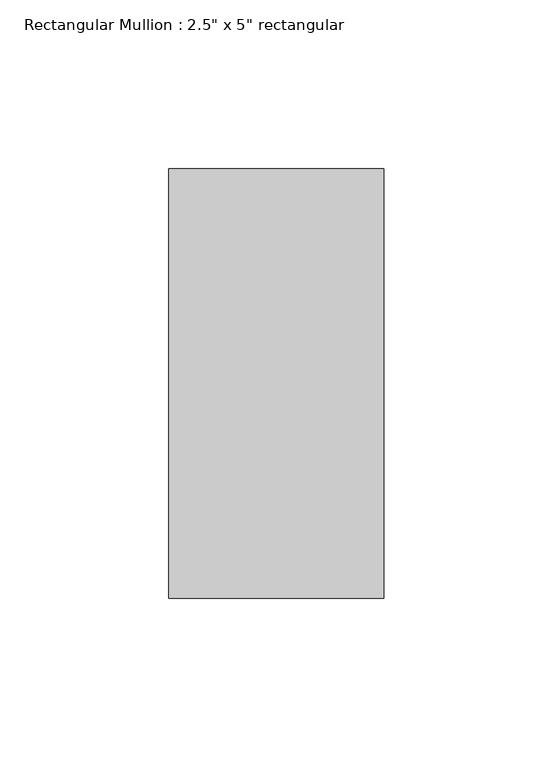
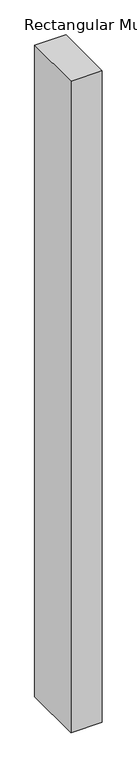
"""IFC4 building model written with IfcOpenShell, lengths in millimetres: member geometry."""

from ifc_helpers import new_model, si_unit, frame, origin, place, context, project, spatial, polyline, outline, extrude, source, transform, mapped, element, save


def member_d08ad361(model_context):
    return source(origin(), model_context, "Body", "SweptSolid", [
        extrude(outline(polyline([(0.0, 63.5), (0.0, -63.5), (-63.5, -63.5), (-63.5, 63.5), (0.0, 63.5)])), frame((0.0, 0.0, -1397.2284812), z_axis=(0.0, 0.0, 1.0), x_axis=(1.0, 0.0, 0.0)), (0.0, 0.0, 1.0), 1397.2284812),
    ])


if __name__ == "__main__":
    model = new_model("IFC4")
    model_context = context("Model", 3, world=origin())
    ifc_project = project(units=[si_unit("LENGTHUNIT", "METRE", prefix="MILLI")], contexts=[model_context])
    site = spatial("IfcSite", under=ifc_project)
    building = spatial("IfcBuilding", under=site)
    placement = place(None, origin())
    member_shape = member_d08ad361(model_context)
    element("IfcMember", 1, ObjectType="Rectangular Mullion : 2.5\" x 5\" rectangular", at=placement, inside=building, context=model_context, shape_type="MappedRepresentation", body=[
        mapped(member_shape, transform((0.0, 0.0, 0.0), x_axis=(1.0, 0.0, 0.0), y_axis=(0.0, 1.0, 0.0), z_axis=(0.0, 0.0, 1.0))),
    ])
    save(model, "model.ifc")

# Revit data of these elements
# Type "Rectangular Mullion : 2.5\" x 5\" rectangular"
#   built-in parameter 1007304 = 0.416667 (stored number, unit not read)
#   built-in parameter 1007301 = 0.104167 (stored number, unit not read)
#   built-in parameter 1007300 = 0.104167 (stored number, unit not read)
# Element 1 (IfcMember, "Rectangular Mullion : 2.5\" x 5\" rectangular")
#   Materials on its faces: "Aluminum"
# Materials
#   "Aluminum": class "Metal", colour RGB 247 247 247, transparency 0, Description = "Aluminum 6061", Cost = 0
